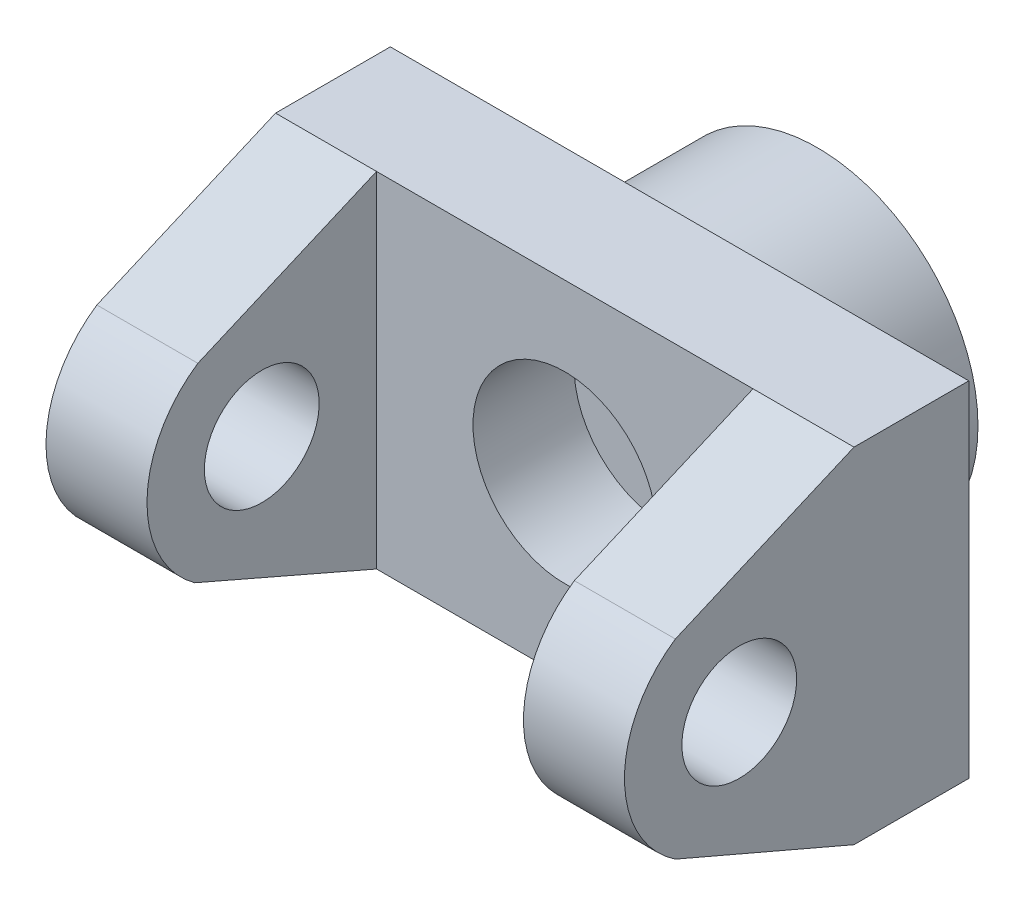
ISO-10303-21;
HEADER;
FILE_DESCRIPTION(('STEP AP214'),'2;1');
FILE_NAME('part.step','',(''),(''),'','','');
FILE_SCHEMA(('AUTOMOTIVE_DESIGN { 1 0 10303 214 1 1 1 1 }'));
ENDSEC;
DATA;
#1=APPLICATION_CONTEXT('core data for automotive mechanical design processes');
#2=APPLICATION_PROTOCOL_DEFINITION('international standard','automotive_design',2000,#1);
#3=PRODUCT_CONTEXT('',#1,'mechanical');
#4=PRODUCT('Part','Part','',(#3));
#5=PRODUCT_RELATED_PRODUCT_CATEGORY('part','',(#4));
#6=PRODUCT_DEFINITION_FORMATION('','',#4);
#7=PRODUCT_DEFINITION_CONTEXT('part definition',#1,'design');
#8=PRODUCT_DEFINITION('design','',#6,#7);
#9=PRODUCT_DEFINITION_SHAPE('','',#8);
#10=(LENGTH_UNIT() NAMED_UNIT(*) SI_UNIT(.MILLI.,.METRE.));
#11=(NAMED_UNIT(*) PLANE_ANGLE_UNIT() SI_UNIT($,.RADIAN.));
#12=(NAMED_UNIT(*) SI_UNIT($,.STERADIAN.) SOLID_ANGLE_UNIT());
#13=UNCERTAINTY_MEASURE_WITH_UNIT(LENGTH_MEASURE(1.E-05),#10,'distance_accuracy_value','');
#14=(GEOMETRIC_REPRESENTATION_CONTEXT(3) GLOBAL_UNCERTAINTY_ASSIGNED_CONTEXT((#13)) GLOBAL_UNIT_ASSIGNED_CONTEXT((#10,
#11,#12)) REPRESENTATION_CONTEXT('',''));
#15=CARTESIAN_POINT('',(0.,0.,0.));
#16=DIRECTION('',(0.,0.,1.));
#17=DIRECTION('',(1.,0.,0.));
#18=AXIS2_PLACEMENT_3D('',#15,#16,#17);
#19=CARTESIAN_POINT('',(0.,0.,25.));
#20=DIRECTION('',(0.,0.,1.));
#21=DIRECTION('',(1.,0.,0.));
#22=AXIS2_PLACEMENT_3D('',#19,#20,#21);
#23=PLANE('',#22);
#24=CARTESIAN_POINT('',(63.,37.7364408388751,25.));
#25=DIRECTION('',(0.,0.,1.));
#26=DIRECTION('',(1.,0.,0.));
#27=AXIS2_PLACEMENT_3D('',#24,#25,#26);
#28=CIRCLE('',#27,20.);
#29=CARTESIAN_POINT('',(83.,37.7364408388751,25.));
#30=VERTEX_POINT('',#29);
#31=EDGE_CURVE('E464',#30,#30,#28,.T.);
#32=ORIENTED_EDGE('',*,*,#31,.F.);
#33=EDGE_LOOP('',(#32));
#34=FACE_BOUND('',#33,.T.);
#35=DIRECTION('',(-1.,0.,0.));
#36=VECTOR('',#35,1.);
#37=CARTESIAN_POINT('',(126.,75.,25.));
#38=LINE('',#37,#36);
#39=CARTESIAN_POINT('',(104.,75.,25.));
#40=VERTEX_POINT('',#39);
#41=CARTESIAN_POINT('',(22.,75.,25.));
#42=VERTEX_POINT('',#41);
#43=EDGE_CURVE('E189',#40,#42,#38,.T.);
#44=ORIENTED_EDGE('',*,*,#43,.T.);
#45=DIRECTION('',(0.,-1.,0.));
#46=VECTOR('',#45,1.);
#47=CARTESIAN_POINT('',(22.,75.,25.));
#48=LINE('',#47,#46);
#49=CARTESIAN_POINT('',(22.,0.,25.));
#50=VERTEX_POINT('',#49);
#51=EDGE_CURVE('E62',#42,#50,#48,.T.);
#52=ORIENTED_EDGE('',*,*,#51,.T.);
#53=DIRECTION('',(1.,0.,0.));
#54=VECTOR('',#53,1.);
#55=CARTESIAN_POINT('',(0.,0.,25.));
#56=LINE('',#55,#54);
#57=CARTESIAN_POINT('',(104.,0.,25.));
#58=VERTEX_POINT('',#57);
#59=EDGE_CURVE('E186',#50,#58,#56,.T.);
#60=ORIENTED_EDGE('',*,*,#59,.T.);
#61=DIRECTION('',(0.,1.,0.));
#62=VECTOR('',#61,1.);
#63=CARTESIAN_POINT('',(104.,75.,25.));
#64=LINE('',#63,#62);
#65=EDGE_CURVE('E167',#58,#40,#64,.T.);
#66=ORIENTED_EDGE('',*,*,#65,.T.);
#67=EDGE_LOOP('',(#44,#52,#60,#66));
#68=FACE_BOUND('',#67,.T.);
#69=ADVANCED_FACE('F44',(#34,#68),#23,.T.);
#70=CARTESIAN_POINT('',(0.,75.,25.));
#71=DIRECTION('',(1.,0.,0.));
#72=DIRECTION('',(0.,0.,-1.));
#73=AXIS2_PLACEMENT_3D('',#70,#71,#72);
#74=PLANE('',#73);
#75=CARTESIAN_POINT('',(0.,37.5,50.));
#76=DIRECTION('',(-1.,0.,0.));
#77=DIRECTION('',(0.,0.,1.));
#78=AXIS2_PLACEMENT_3D('',#75,#76,#77);
#79=CIRCLE('',#78,12.5);
#80=CARTESIAN_POINT('',(0.,37.5,62.5));
#81=VERTEX_POINT('',#80);
#82=EDGE_CURVE('E453',#81,#81,#79,.T.);
#83=ORIENTED_EDGE('',*,*,#82,.F.);
#84=EDGE_LOOP('',(#83));
#85=FACE_BOUND('',#84,.T.);
#86=DIRECTION('',(0.,-1.,0.));
#87=VECTOR('',#86,1.);
#88=CARTESIAN_POINT('',(0.,75.,0.));
#89=LINE('',#88,#87);
#90=CARTESIAN_POINT('',(0.,75.,0.));
#91=VERTEX_POINT('',#90);
#92=CARTESIAN_POINT('',(0.,0.,0.));
#93=VERTEX_POINT('',#92);
#94=EDGE_CURVE('E182',#91,#93,#89,.T.);
#95=ORIENTED_EDGE('',*,*,#94,.T.);
#96=DIRECTION('',(0.,0.,-1.));
#97=VECTOR('',#96,1.);
#98=CARTESIAN_POINT('',(0.,0.,25.));
#99=LINE('',#98,#97);
#100=CARTESIAN_POINT('',(0.,0.,25.));
#101=VERTEX_POINT('',#100);
#102=EDGE_CURVE('E47',#101,#93,#99,.T.);
#103=ORIENTED_EDGE('',*,*,#102,.F.);
#104=DIRECTION('',(0.,0.398506393756268,0.917165554376839));
#105=VECTOR('',#104,1.);
#106=CARTESIAN_POINT('',(0.,0.,25.));
#107=LINE('',#106,#105);
#108=CARTESIAN_POINT('',(0.,17.2060408228928,64.5998363318877));
#109=VERTEX_POINT('',#108);
#110=EDGE_CURVE('E153',#101,#109,#107,.T.);
#111=ORIENTED_EDGE('',*,*,#110,.T.);
#112=CARTESIAN_POINT('',(0.,37.5,50.));
#113=DIRECTION('',(-1.,0.,0.));
#114=DIRECTION('',(0.,0.,1.));
#115=AXIS2_PLACEMENT_3D('',#112,#113,#114);
#116=CIRCLE('',#115,25.);
#117=CARTESIAN_POINT('',(0.,58.2668408548574,63.9189913754203));
#118=VERTEX_POINT('',#117);
#119=EDGE_CURVE('E128',#109,#118,#116,.T.);
#120=ORIENTED_EDGE('',*,*,#119,.T.);
#121=DIRECTION('',(0.,0.394987764739422,-0.918686380494538));
#122=VECTOR('',#121,1.);
#123=CARTESIAN_POINT('',(0.,75.,25.));
#124=LINE('',#123,#122);
#125=CARTESIAN_POINT('',(0.,75.,25.));
#126=VERTEX_POINT('',#125);
#127=EDGE_CURVE('E151',#118,#126,#124,.T.);
#128=ORIENTED_EDGE('',*,*,#127,.T.);
#129=DIRECTION('',(0.,0.,-1.));
#130=VECTOR('',#129,1.);
#131=CARTESIAN_POINT('',(0.,75.,25.));
#132=LINE('',#131,#130);
#133=EDGE_CURVE('E194',#126,#91,#132,.T.);
#134=ORIENTED_EDGE('',*,*,#133,.T.);
#135=EDGE_LOOP('',(#95,#103,#111,#120,#128,#134));
#136=FACE_BOUND('',#135,.T.);
#137=ADVANCED_FACE('F50',(#85,#136),#74,.F.);
#138=CARTESIAN_POINT('',(0.,0.,25.));
#139=DIRECTION('',(0.,1.,0.));
#140=DIRECTION('',(0.,0.,1.));
#141=AXIS2_PLACEMENT_3D('',#138,#139,#140);
#142=PLANE('',#141);
#143=DIRECTION('',(1.,0.,0.));
#144=VECTOR('',#143,1.);
#145=CARTESIAN_POINT('',(0.,0.,0.));
#146=LINE('',#145,#144);
#147=CARTESIAN_POINT('',(126.,0.,0.));
#148=VERTEX_POINT('',#147);
#149=EDGE_CURVE('E196',#93,#148,#146,.T.);
#150=ORIENTED_EDGE('',*,*,#149,.T.);
#151=DIRECTION('',(0.,0.,-1.));
#152=VECTOR('',#151,1.);
#153=CARTESIAN_POINT('',(126.,0.,25.));
#154=LINE('',#153,#152);
#155=CARTESIAN_POINT('',(126.,0.,25.));
#156=VERTEX_POINT('',#155);
#157=EDGE_CURVE('E207',#156,#148,#154,.T.);
#158=ORIENTED_EDGE('',*,*,#157,.F.);
#159=DIRECTION('',(1.,0.,0.));
#160=VECTOR('',#159,1.);
#161=CARTESIAN_POINT('',(104.,0.,25.));
#162=LINE('',#161,#160);
#163=EDGE_CURVE('E181',#58,#156,#162,.T.);
#164=ORIENTED_EDGE('',*,*,#163,.F.);
#165=ORIENTED_EDGE('',*,*,#59,.F.);
#166=EDGE_CURVE('E139',#101,#50,#56,.T.);
#167=ORIENTED_EDGE('',*,*,#166,.F.);
#168=ORIENTED_EDGE('',*,*,#102,.T.);
#169=EDGE_LOOP('',(#150,#158,#164,#165,#167,#168));
#170=FACE_BOUND('',#169,.T.);
#171=ADVANCED_FACE('F211',(#170),#142,.F.);
#172=CARTESIAN_POINT('',(126.,0.,25.));
#173=DIRECTION('',(-1.,0.,0.));
#174=DIRECTION('',(0.,0.,1.));
#175=AXIS2_PLACEMENT_3D('',#172,#173,#174);
#176=PLANE('',#175);
#177=CARTESIAN_POINT('',(126.,37.5,50.));
#178=DIRECTION('',(1.,0.,0.));
#179=DIRECTION('',(0.,0.,-1.));
#180=AXIS2_PLACEMENT_3D('',#177,#178,#179);
#181=CIRCLE('',#180,12.5);
#182=CARTESIAN_POINT('',(126.,37.5,37.5));
#183=VERTEX_POINT('',#182);
#184=EDGE_CURVE('E454',#183,#183,#181,.T.);
#185=ORIENTED_EDGE('',*,*,#184,.F.);
#186=EDGE_LOOP('',(#185));
#187=FACE_BOUND('',#186,.T.);
#188=DIRECTION('',(0.,1.,0.));
#189=VECTOR('',#188,1.);
#190=CARTESIAN_POINT('',(126.,0.,0.));
#191=LINE('',#190,#189);
#192=CARTESIAN_POINT('',(126.,75.,0.));
#193=VERTEX_POINT('',#192);
#194=EDGE_CURVE('E199',#148,#193,#191,.T.);
#195=ORIENTED_EDGE('',*,*,#194,.T.);
#196=DIRECTION('',(0.,0.,-1.));
#197=VECTOR('',#196,1.);
#198=CARTESIAN_POINT('',(126.,75.,25.));
#199=LINE('',#198,#197);
#200=CARTESIAN_POINT('',(126.,75.,25.));
#201=VERTEX_POINT('',#200);
#202=EDGE_CURVE('E202',#201,#193,#199,.T.);
#203=ORIENTED_EDGE('',*,*,#202,.F.);
#204=DIRECTION('',(0.,-0.394987764739422,0.918686380494538));
#205=VECTOR('',#204,1.);
#206=CARTESIAN_POINT('',(126.,75.,25.));
#207=LINE('',#206,#205);
#208=CARTESIAN_POINT('',(126.,58.2668408548574,63.9189913754203));
#209=VERTEX_POINT('',#208);
#210=EDGE_CURVE('E156',#201,#209,#207,.T.);
#211=ORIENTED_EDGE('',*,*,#210,.T.);
#212=CARTESIAN_POINT('',(126.,37.5,50.));
#213=DIRECTION('',(1.,0.,0.));
#214=DIRECTION('',(0.,0.,-1.));
#215=AXIS2_PLACEMENT_3D('',#212,#213,#214);
#216=CIRCLE('',#215,25.);
#217=CARTESIAN_POINT('',(126.,16.7331591451426,63.9189913754203));
#218=VERTEX_POINT('',#217);
#219=EDGE_CURVE('E176',#209,#218,#216,.T.);
#220=ORIENTED_EDGE('',*,*,#219,.T.);
#221=DIRECTION('',(0.,-0.394987764739422,-0.918686380494538));
#222=VECTOR('',#221,1.);
#223=CARTESIAN_POINT('',(126.,0.,25.));
#224=LINE('',#223,#222);
#225=EDGE_CURVE('E165',#218,#156,#224,.T.);
#226=ORIENTED_EDGE('',*,*,#225,.T.);
#227=ORIENTED_EDGE('',*,*,#157,.T.);
#228=EDGE_LOOP('',(#195,#203,#211,#220,#226,#227));
#229=FACE_BOUND('',#228,.T.);
#230=ADVANCED_FACE('F223',(#187,#229),#176,.F.);
#231=CARTESIAN_POINT('',(126.,75.,25.));
#232=DIRECTION('',(0.,-1.,0.));
#233=DIRECTION('',(0.,0.,-1.));
#234=AXIS2_PLACEMENT_3D('',#231,#232,#233);
#235=PLANE('',#234);
#236=DIRECTION('',(-1.,0.,0.));
#237=VECTOR('',#236,1.);
#238=CARTESIAN_POINT('',(126.,75.,0.));
#239=LINE('',#238,#237);
#240=EDGE_CURVE('E200',#193,#91,#239,.T.);
#241=ORIENTED_EDGE('',*,*,#240,.T.);
#242=ORIENTED_EDGE('',*,*,#133,.F.);
#243=DIRECTION('',(-1.,0.,0.));
#244=VECTOR('',#243,1.);
#245=CARTESIAN_POINT('',(22.,75.,25.));
#246=LINE('',#245,#244);
#247=EDGE_CURVE('E68',#42,#126,#246,.T.);
#248=ORIENTED_EDGE('',*,*,#247,.F.);
#249=ORIENTED_EDGE('',*,*,#43,.F.);
#250=EDGE_CURVE('E188',#201,#40,#38,.T.);
#251=ORIENTED_EDGE('',*,*,#250,.F.);
#252=ORIENTED_EDGE('',*,*,#202,.T.);
#253=EDGE_LOOP('',(#241,#242,#248,#249,#251,#252));
#254=FACE_BOUND('',#253,.T.);
#255=ADVANCED_FACE('F221',(#254),#235,.F.);
#256=CARTESIAN_POINT('',(0.,0.,0.));
#257=DIRECTION('',(0.,0.,1.));
#258=DIRECTION('',(1.,0.,0.));
#259=AXIS2_PLACEMENT_3D('',#256,#257,#258);
#260=PLANE('',#259);
#261=CARTESIAN_POINT('',(63.,37.5,0.));
#262=DIRECTION('',(0.,0.,-1.));
#263=DIRECTION('',(-1.,0.,0.));
#264=AXIS2_PLACEMENT_3D('',#261,#262,#263);
#265=CIRCLE('',#264,35.);
#266=CARTESIAN_POINT('',(28.,37.5,0.));
#267=VERTEX_POINT('',#266);
#268=EDGE_CURVE('E11',#267,#267,#265,.T.);
#269=ORIENTED_EDGE('',*,*,#268,.F.);
#270=EDGE_LOOP('',(#269));
#271=FACE_BOUND('',#270,.T.);
#272=ORIENTED_EDGE('',*,*,#94,.F.);
#273=ORIENTED_EDGE('',*,*,#240,.F.);
#274=ORIENTED_EDGE('',*,*,#194,.F.);
#275=ORIENTED_EDGE('',*,*,#149,.F.);
#276=EDGE_LOOP('',(#272,#273,#274,#275));
#277=FACE_BOUND('',#276,.T.);
#278=ADVANCED_FACE('F218',(#271,#277),#260,.F.);
#279=CARTESIAN_POINT('',(104.,75.,25.));
#280=DIRECTION('',(0.,0.918686380494538,0.394987764739422));
#281=DIRECTION('',(0.,-0.394987764739422,0.918686380494538));
#282=AXIS2_PLACEMENT_3D('',#279,#280,#281);
#283=PLANE('',#282);
#284=ORIENTED_EDGE('',*,*,#210,.F.);
#285=ORIENTED_EDGE('',*,*,#250,.T.);
#286=DIRECTION('',(0.,-0.394987764739422,0.918686380494538));
#287=VECTOR('',#286,1.);
#288=CARTESIAN_POINT('',(104.,75.,25.));
#289=LINE('',#288,#287);
#290=CARTESIAN_POINT('',(104.,58.2668408548574,63.9189913754203));
#291=VERTEX_POINT('',#290);
#292=EDGE_CURVE('E159',#40,#291,#289,.T.);
#293=ORIENTED_EDGE('',*,*,#292,.T.);
#294=DIRECTION('',(1.,0.,0.));
#295=VECTOR('',#294,1.);
#296=CARTESIAN_POINT('',(104.,58.2668408548574,63.9189913754203));
#297=LINE('',#296,#295);
#298=EDGE_CURVE('E173',#291,#209,#297,.T.);
#299=ORIENTED_EDGE('',*,*,#298,.T.);
#300=EDGE_LOOP('',(#284,#285,#293,#299));
#301=FACE_BOUND('',#300,.T.);
#302=ADVANCED_FACE('F224',(#301),#283,.T.);
#303=CARTESIAN_POINT('',(104.,0.,25.));
#304=DIRECTION('',(0.,-0.918686380494538,0.394987764739422));
#305=DIRECTION('',(0.,-0.394987764739422,-0.918686380494538));
#306=AXIS2_PLACEMENT_3D('',#303,#304,#305);
#307=PLANE('',#306);
#308=ORIENTED_EDGE('',*,*,#225,.F.);
#309=DIRECTION('',(1.,0.,0.));
#310=VECTOR('',#309,1.);
#311=CARTESIAN_POINT('',(104.,16.7331591451426,63.9189913754203));
#312=LINE('',#311,#310);
#313=CARTESIAN_POINT('',(104.,16.7331591451426,63.9189913754203));
#314=VERTEX_POINT('',#313);
#315=EDGE_CURVE('E183',#314,#218,#312,.T.);
#316=ORIENTED_EDGE('',*,*,#315,.F.);
#317=DIRECTION('',(0.,-0.394987764739422,-0.918686380494538));
#318=VECTOR('',#317,1.);
#319=CARTESIAN_POINT('',(104.,0.,25.));
#320=LINE('',#319,#318);
#321=EDGE_CURVE('E170',#314,#58,#320,.T.);
#322=ORIENTED_EDGE('',*,*,#321,.T.);
#323=ORIENTED_EDGE('',*,*,#163,.T.);
#324=EDGE_LOOP('',(#308,#316,#322,#323));
#325=FACE_BOUND('',#324,.T.);
#326=ADVANCED_FACE('F234',(#325),#307,.T.);
#327=CARTESIAN_POINT('',(104.,37.5,50.));
#328=DIRECTION('',(1.,0.,0.));
#329=DIRECTION('',(0.,0.,-1.));
#330=AXIS2_PLACEMENT_3D('',#327,#328,#329);
#331=CYLINDRICAL_SURFACE('',#330,25.);
#332=ORIENTED_EDGE('',*,*,#219,.F.);
#333=ORIENTED_EDGE('',*,*,#298,.F.);
#334=CARTESIAN_POINT('',(104.,37.5,50.));
#335=DIRECTION('',(1.,0.,0.));
#336=DIRECTION('',(0.,0.,-1.));
#337=AXIS2_PLACEMENT_3D('',#334,#335,#336);
#338=CIRCLE('',#337,25.);
#339=EDGE_CURVE('E161',#291,#314,#338,.T.);
#340=ORIENTED_EDGE('',*,*,#339,.T.);
#341=ORIENTED_EDGE('',*,*,#315,.T.);
#342=EDGE_LOOP('',(#332,#333,#340,#341));
#343=FACE_BOUND('',#342,.T.);
#344=ADVANCED_FACE('F240',(#343),#331,.T.);
#345=CARTESIAN_POINT('',(104.,37.5,50.));
#346=DIRECTION('',(1.,0.,0.));
#347=DIRECTION('',(0.,0.,-1.));
#348=AXIS2_PLACEMENT_3D('',#345,#346,#347);
#349=PLANE('',#348);
#350=CARTESIAN_POINT('',(104.,37.5,50.));
#351=DIRECTION('',(1.,0.,0.));
#352=DIRECTION('',(0.,0.,-1.));
#353=AXIS2_PLACEMENT_3D('',#350,#351,#352);
#354=CIRCLE('',#353,12.5);
#355=CARTESIAN_POINT('',(104.,37.5,37.5));
#356=VERTEX_POINT('',#355);
#357=EDGE_CURVE('E448',#356,#356,#354,.T.);
#358=ORIENTED_EDGE('',*,*,#357,.T.);
#359=EDGE_LOOP('',(#358));
#360=FACE_BOUND('',#359,.T.);
#361=ORIENTED_EDGE('',*,*,#292,.F.);
#362=ORIENTED_EDGE('',*,*,#65,.F.);
#363=ORIENTED_EDGE('',*,*,#321,.F.);
#364=ORIENTED_EDGE('',*,*,#339,.F.);
#365=EDGE_LOOP('',(#361,#362,#363,#364));
#366=FACE_BOUND('',#365,.T.);
#367=ADVANCED_FACE('F229',(#360,#366),#349,.F.);
#368=CARTESIAN_POINT('',(22.,75.,25.));
#369=DIRECTION('',(0.,0.918686380494538,0.394987764739422));
#370=DIRECTION('',(0.,-0.394987764739422,0.918686380494538));
#371=AXIS2_PLACEMENT_3D('',#368,#369,#370);
#372=PLANE('',#371);
#373=ORIENTED_EDGE('',*,*,#127,.F.);
#374=DIRECTION('',(-1.,0.,0.));
#375=VECTOR('',#374,1.);
#376=CARTESIAN_POINT('',(22.,58.2668408548574,63.9189913754203));
#377=LINE('',#376,#375);
#378=CARTESIAN_POINT('',(22.,58.2668408548574,63.9189913754203));
#379=VERTEX_POINT('',#378);
#380=EDGE_CURVE('E133',#379,#118,#377,.T.);
#381=ORIENTED_EDGE('',*,*,#380,.F.);
#382=DIRECTION('',(0.,0.394987764739422,-0.918686380494538));
#383=VECTOR('',#382,1.);
#384=CARTESIAN_POINT('',(22.,75.,25.));
#385=LINE('',#384,#383);
#386=EDGE_CURVE('E147',#379,#42,#385,.T.);
#387=ORIENTED_EDGE('',*,*,#386,.T.);
#388=ORIENTED_EDGE('',*,*,#247,.T.);
#389=EDGE_LOOP('',(#373,#381,#387,#388));
#390=FACE_BOUND('',#389,.T.);
#391=ADVANCED_FACE('F244',(#390),#372,.T.);
#392=CARTESIAN_POINT('',(22.,37.5,50.));
#393=DIRECTION('',(-1.,0.,0.));
#394=DIRECTION('',(0.,0.,1.));
#395=AXIS2_PLACEMENT_3D('',#392,#393,#394);
#396=CYLINDRICAL_SURFACE('',#395,25.);
#397=ORIENTED_EDGE('',*,*,#119,.F.);
#398=DIRECTION('',(-1.,0.,0.));
#399=VECTOR('',#398,1.);
#400=CARTESIAN_POINT('',(22.,17.2060408228928,64.5998363318877));
#401=LINE('',#400,#399);
#402=CARTESIAN_POINT('',(22.,17.2060408228928,64.5998363318877));
#403=VERTEX_POINT('',#402);
#404=EDGE_CURVE('E121',#403,#109,#401,.T.);
#405=ORIENTED_EDGE('',*,*,#404,.F.);
#406=CARTESIAN_POINT('',(22.,37.5,50.));
#407=DIRECTION('',(-1.,0.,0.));
#408=DIRECTION('',(0.,0.,1.));
#409=AXIS2_PLACEMENT_3D('',#406,#407,#408);
#410=CIRCLE('',#409,25.);
#411=EDGE_CURVE('E129',#403,#379,#410,.T.);
#412=ORIENTED_EDGE('',*,*,#411,.T.);
#413=ORIENTED_EDGE('',*,*,#380,.T.);
#414=EDGE_LOOP('',(#397,#405,#412,#413));
#415=FACE_BOUND('',#414,.T.);
#416=ADVANCED_FACE('F127',(#415),#396,.T.);
#417=CARTESIAN_POINT('',(22.,0.,25.));
#418=DIRECTION('',(0.,-0.917165554376839,0.398506393756268));
#419=DIRECTION('',(0.,-0.398506393756268,-0.917165554376839));
#420=AXIS2_PLACEMENT_3D('',#417,#418,#419);
#421=PLANE('',#420);
#422=ORIENTED_EDGE('',*,*,#110,.F.);
#423=ORIENTED_EDGE('',*,*,#166,.T.);
#424=DIRECTION('',(0.,0.398506393756268,0.917165554376839));
#425=VECTOR('',#424,1.);
#426=CARTESIAN_POINT('',(22.,0.,25.));
#427=LINE('',#426,#425);
#428=EDGE_CURVE('E136',#50,#403,#427,.T.);
#429=ORIENTED_EDGE('',*,*,#428,.T.);
#430=ORIENTED_EDGE('',*,*,#404,.T.);
#431=EDGE_LOOP('',(#422,#423,#429,#430));
#432=FACE_BOUND('',#431,.T.);
#433=ADVANCED_FACE('F137',(#432),#421,.T.);
#434=CARTESIAN_POINT('',(22.,37.5,50.));
#435=DIRECTION('',(-1.,0.,0.));
#436=DIRECTION('',(0.,0.,1.));
#437=AXIS2_PLACEMENT_3D('',#434,#435,#436);
#438=PLANE('',#437);
#439=CARTESIAN_POINT('',(22.,37.5,50.));
#440=DIRECTION('',(-1.,0.,0.));
#441=DIRECTION('',(0.,0.,1.));
#442=AXIS2_PLACEMENT_3D('',#439,#440,#441);
#443=CIRCLE('',#442,12.5);
#444=CARTESIAN_POINT('',(22.,37.5,62.5));
#445=VERTEX_POINT('',#444);
#446=EDGE_CURVE('E459',#445,#445,#443,.T.);
#447=ORIENTED_EDGE('',*,*,#446,.T.);
#448=EDGE_LOOP('',(#447));
#449=FACE_BOUND('',#448,.T.);
#450=ORIENTED_EDGE('',*,*,#386,.F.);
#451=ORIENTED_EDGE('',*,*,#411,.F.);
#452=ORIENTED_EDGE('',*,*,#428,.F.);
#453=ORIENTED_EDGE('',*,*,#51,.F.);
#454=EDGE_LOOP('',(#450,#451,#452,#453));
#455=FACE_BOUND('',#454,.T.);
#456=ADVANCED_FACE('F144',(#449,#455),#438,.F.);
#457=CARTESIAN_POINT('',(63.,37.7364408388751,3.));
#458=DIRECTION('',(0.,0.,1.));
#459=DIRECTION('',(1.,0.,0.));
#460=AXIS2_PLACEMENT_3D('',#457,#458,#459);
#461=CYLINDRICAL_SURFACE('',#460,20.);
#462=CARTESIAN_POINT('',(63.,37.7364408388751,3.));
#463=DIRECTION('',(0.,0.,1.));
#464=DIRECTION('',(1.,0.,0.));
#465=AXIS2_PLACEMENT_3D('',#462,#463,#464);
#466=CIRCLE('',#465,20.);
#467=CARTESIAN_POINT('',(83.,37.7364408388751,3.));
#468=VERTEX_POINT('',#467);
#469=EDGE_CURVE('E155',#468,#468,#466,.T.);
#470=ORIENTED_EDGE('',*,*,#469,.F.);
#471=EDGE_LOOP('',(#470));
#472=FACE_BOUND('',#471,.T.);
#473=ORIENTED_EDGE('',*,*,#31,.T.);
#474=EDGE_LOOP('',(#473));
#475=FACE_BOUND('',#474,.T.);
#476=ADVANCED_FACE('F309',(#472,#475),#461,.F.);
#477=CARTESIAN_POINT('',(63.,37.7364408388751,3.));
#478=DIRECTION('',(0.,0.,1.));
#479=DIRECTION('',(1.,0.,0.));
#480=AXIS2_PLACEMENT_3D('',#477,#478,#479);
#481=PLANE('',#480);
#482=ORIENTED_EDGE('',*,*,#469,.T.);
#483=EDGE_LOOP('',(#482));
#484=FACE_BOUND('',#483,.T.);
#485=ADVANCED_FACE('F322',(#484),#481,.T.);
#486=CARTESIAN_POINT('',(63.,37.5,-30.));
#487=DIRECTION('',(0.,0.,1.));
#488=DIRECTION('',(1.,0.,0.));
#489=AXIS2_PLACEMENT_3D('',#486,#487,#488);
#490=CYLINDRICAL_SURFACE('',#489,35.);
#491=CARTESIAN_POINT('',(63.,37.5,-30.));
#492=DIRECTION('',(0.,0.,-1.));
#493=DIRECTION('',(-1.,0.,0.));
#494=AXIS2_PLACEMENT_3D('',#491,#492,#493);
#495=CIRCLE('',#494,35.);
#496=CARTESIAN_POINT('',(28.,37.5,-30.));
#497=VERTEX_POINT('',#496);
#498=EDGE_CURVE('E463',#497,#497,#495,.T.);
#499=ORIENTED_EDGE('',*,*,#498,.F.);
#500=EDGE_LOOP('',(#499));
#501=FACE_BOUND('',#500,.T.);
#502=ORIENTED_EDGE('',*,*,#268,.T.);
#503=EDGE_LOOP('',(#502));
#504=FACE_BOUND('',#503,.T.);
#505=ADVANCED_FACE('F331',(#501,#504),#490,.T.);
#506=CARTESIAN_POINT('',(63.,37.5,-30.));
#507=DIRECTION('',(0.,0.,-1.));
#508=DIRECTION('',(-1.,0.,0.));
#509=AXIS2_PLACEMENT_3D('',#506,#507,#508);
#510=PLANE('',#509);
#511=ORIENTED_EDGE('',*,*,#498,.T.);
#512=EDGE_LOOP('',(#511));
#513=FACE_BOUND('',#512,.T.);
#514=ADVANCED_FACE('F343',(#513),#510,.T.);
#515=CARTESIAN_POINT('',(22.,37.5,50.));
#516=DIRECTION('',(-1.,0.,0.));
#517=DIRECTION('',(0.,0.,1.));
#518=AXIS2_PLACEMENT_3D('',#515,#516,#517);
#519=CYLINDRICAL_SURFACE('',#518,12.5);
#520=ORIENTED_EDGE('',*,*,#446,.F.);
#521=EDGE_LOOP('',(#520));
#522=FACE_BOUND('',#521,.T.);
#523=ORIENTED_EDGE('',*,*,#82,.T.);
#524=EDGE_LOOP('',(#523));
#525=FACE_BOUND('',#524,.T.);
#526=ADVANCED_FACE('F357',(#522,#525),#519,.F.);
#527=CARTESIAN_POINT('',(104.,37.5,50.));
#528=DIRECTION('',(1.,0.,0.));
#529=DIRECTION('',(0.,0.,-1.));
#530=AXIS2_PLACEMENT_3D('',#527,#528,#529);
#531=CYLINDRICAL_SURFACE('',#530,12.5);
#532=ORIENTED_EDGE('',*,*,#357,.F.);
#533=EDGE_LOOP('',(#532));
#534=FACE_BOUND('',#533,.T.);
#535=ORIENTED_EDGE('',*,*,#184,.T.);
#536=EDGE_LOOP('',(#535));
#537=FACE_BOUND('',#536,.T.);
#538=ADVANCED_FACE('F368',(#534,#537),#531,.F.);
#539=CLOSED_SHELL('',(#69,#137,#171,#230,#255,#278,#302,#326,#344,#367,#391,#416,#433,#456,#476,
#485,#505,#514,#526,#538));
#540=MANIFOLD_SOLID_BREP('B2',#539);
#541=ADVANCED_BREP_SHAPE_REPRESENTATION('',(#18,#540),#14);
#542=SHAPE_DEFINITION_REPRESENTATION(#9,#541);
ENDSEC;
END-ISO-10303-21;
